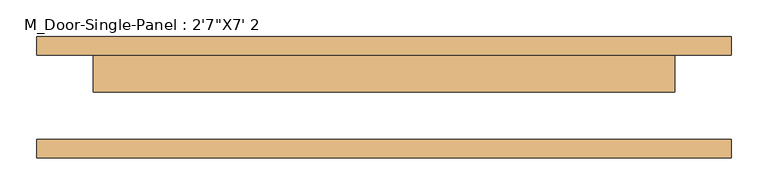
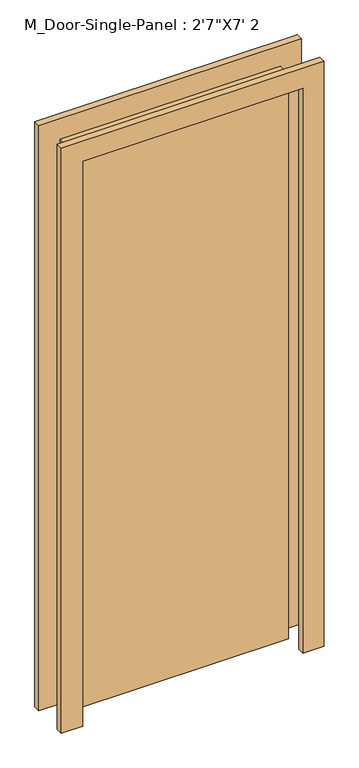
"""IFC4 building model written with IfcOpenShell, lengths in millimetres: door geometry."""

from ifc_helpers import new_model, si_unit, frame, origin, origin_with_axes, place, context, project, spatial, polyline, outline, extrude, source, transform, mapped, element, save


def door_a431d384(model_context):
    return source(origin(), model_context, "Body", "SweptSolid", [
        extrude(outline(polyline([(393.7, 7.15), (-393.7, 7.15), (-393.7, 57.15), (393.7, 57.15), (393.7, 7.15)])), origin_with_axes(), (0.0, 0.0, 1.0), 2133.6),
        extrude(outline(polyline([(2209.8, 469.9), (2209.8, -469.9), (0.0, -469.9), (0.0, -393.7), (2133.6, -393.7), (2133.6, 393.7), (0.0, 393.7), (0.0, 469.9), (2209.8, 469.9)])), frame((0.0, -82.15, 0.0), z_axis=(0.0, 1.0, 0.0), x_axis=(0.0, 0.0, 1.0)), (0.0, 0.0, 1.0), 25.0),
        extrude(outline(polyline([(2209.8, -469.9), (0.0, -469.9), (0.0, -393.7), (2133.6, -393.7), (2133.6, 393.7), (0.0, 393.7), (0.0, 469.9), (2209.8, 469.9), (2209.8, -469.9)])), frame((0.0, 57.15, 0.0), z_axis=(0.0, 1.0, 0.0), x_axis=(0.0, 0.0, 1.0)), (0.0, 0.0, 1.0), 25.0),
    ])


if __name__ == "__main__":
    model = new_model("IFC4")
    model_context = context("Model", 3, world=origin())
    ifc_project = project(units=[si_unit("LENGTHUNIT", "METRE", prefix="MILLI")], contexts=[model_context])
    site = spatial("IfcSite", under=ifc_project)
    building = spatial("IfcBuilding", under=site)
    placement = place(None, origin())
    door_shape = door_a431d384(model_context)
    element("IfcDoor", 1, ObjectType="M_Door-Single-Panel : 2'7\"X7' 2", at=placement, inside=building, context=model_context, shape_type="MappedRepresentation", body=[
        mapped(door_shape, transform((0.0, 0.0, 0.0), x_axis=(1.0, 0.0, 0.0), y_axis=(0.0, 1.0, 0.0), z_axis=(0.0, 0.0, 1.0))),
    ])
    save(model, "model.ifc")

# Revit data of these elements
# Type "M_Door-Single-Panel : 2'7\"X7' 2"
#   Type Mark = "13"
#   Construction Type Id = "DOOR"
#   Assembly Code = "C1020300"
#   Analytic Construction = "Wooden"
#   Thickness = 0' - 1.9685"
#   Thermal Resistance (R) = 2.5876 (h·ft²·°F)/BTU
#   Swing Angle [instance default] = 90.00°
#   Heat Transfer Coefficient (U) = 0.3865 BTU/(h·ft²·°F)
#   Height = 7' - 0"
#   Trim Projection Ext = 0' - 0.98425"
#   Trim Projection Int = 0' - 0.98425"
#   Trim Width = 0' - 3.14961"
#   Width = 2' - 7"
#   Define Thermal Properties by = 1
#   Panel Material = Wood - Birch - Solid Stained Light Low Gloss
#   Trim Material = Paint - Sienna
#   Visual Light Transmittance = 0
#   Solar Heat Gain Coefficient = 0
#   Function = (empty or 0)
#   Wall Closure = (empty or 0)
# Element 1 (IfcDoor, "M_Door-Single-Panel : 2'7\"X7' 2")
#   Materials on its faces: "Paint - Sienna", "Wood - Birch - Solid Stained Light Low Gloss"
# Materials
#   "Wood - Birch - Solid Stained Light Low Gloss": class "Wood", colour RGB 210 159 95, transparency 0, Cost = 0
#   "Paint - Sienna": colour RGB 118 70 51, transparency 0, Cost = 0
